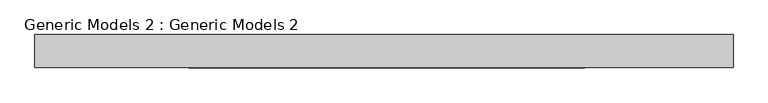
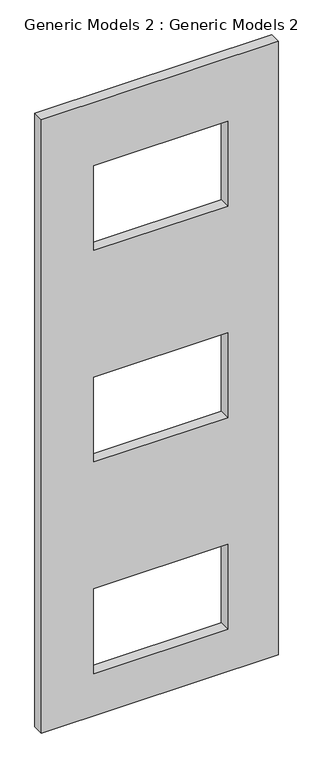
"""IFC4 building model written with IfcOpenShell, lengths in millimetres: proxy geometry, Generic Models 2 : Generic Models 2."""

from ifc_helpers import new_model, si_unit, frame, origin, place, context, project, spatial, polyline, outline, extrude, source, transform, mapped, element, save


def generic_models_2_generic_models_2_e2b5cfd4(model_context):
    return source(origin(), model_context, "Body", "SweptSolid", [
        extrude(outline(polyline([(12192.0, 1674.8824202), (12192.0, -1550.9175798), (3352.8, -1550.9175798), (3352.8, 1674.8824202), (12192.0, 1674.8824202)]), holes=[polyline([(11277.6, 989.0824202), (10058.4, 989.0824202), (10058.4, -839.7175798), (11277.6, -839.7175798), (11277.6, 989.0824202)]), polyline([(8229.6, 989.0824202), (7010.4, 989.0824202), (7010.4, -839.7175798), (8229.6, -839.7175798), (8229.6, 989.0824202)]), polyline([(5181.6, 989.0824202), (3962.4, 989.0824202), (3962.4, -839.7175798), (5181.6, -839.7175798), (5181.6, 989.0824202)])]), frame((0.0, -13103.6402089, 0.0), z_axis=(0.0, 1.0, 0.0), x_axis=(0.0, 0.0, 1.0)), (0.0, 0.0, 1.0), 152.4),
    ])


if __name__ == "__main__":
    model = new_model("IFC4")
    model_context = context("Model", 3, world=origin())
    ifc_project = project(units=[si_unit("LENGTHUNIT", "METRE", prefix="MILLI")], contexts=[model_context])
    site = spatial("IfcSite", under=ifc_project)
    building = spatial("IfcBuilding", under=site)
    placement = place(None, origin())
    generic_models_2_generic_models_2_shape = generic_models_2_generic_models_2_e2b5cfd4(model_context)
    element("IfcBuildingElementProxy", 1, Name="Generic Models 2 : Generic Models 2", ObjectType="Generic Models 2 : Generic Models 2", at=placement, inside=building, context=model_context, shape_type="MappedRepresentation", body=[
        mapped(generic_models_2_generic_models_2_shape, transform((0.0, 0.0, 0.0), x_axis=(1.0, 0.0, 0.0), y_axis=(0.0, 1.0, 0.0), z_axis=(0.0, 0.0, 1.0))),
    ])
    save(model, "model.ifc")

# Revit data of these elements
# Element 1 (IfcBuildingElementProxy, "Generic Models 2 : Generic Models 2")
#   Materials on its faces: "black accent wall"
# Materials
#   "black accent wall": class "Generic", colour RGB 120 120 120, transparency 0, Cost = 0
